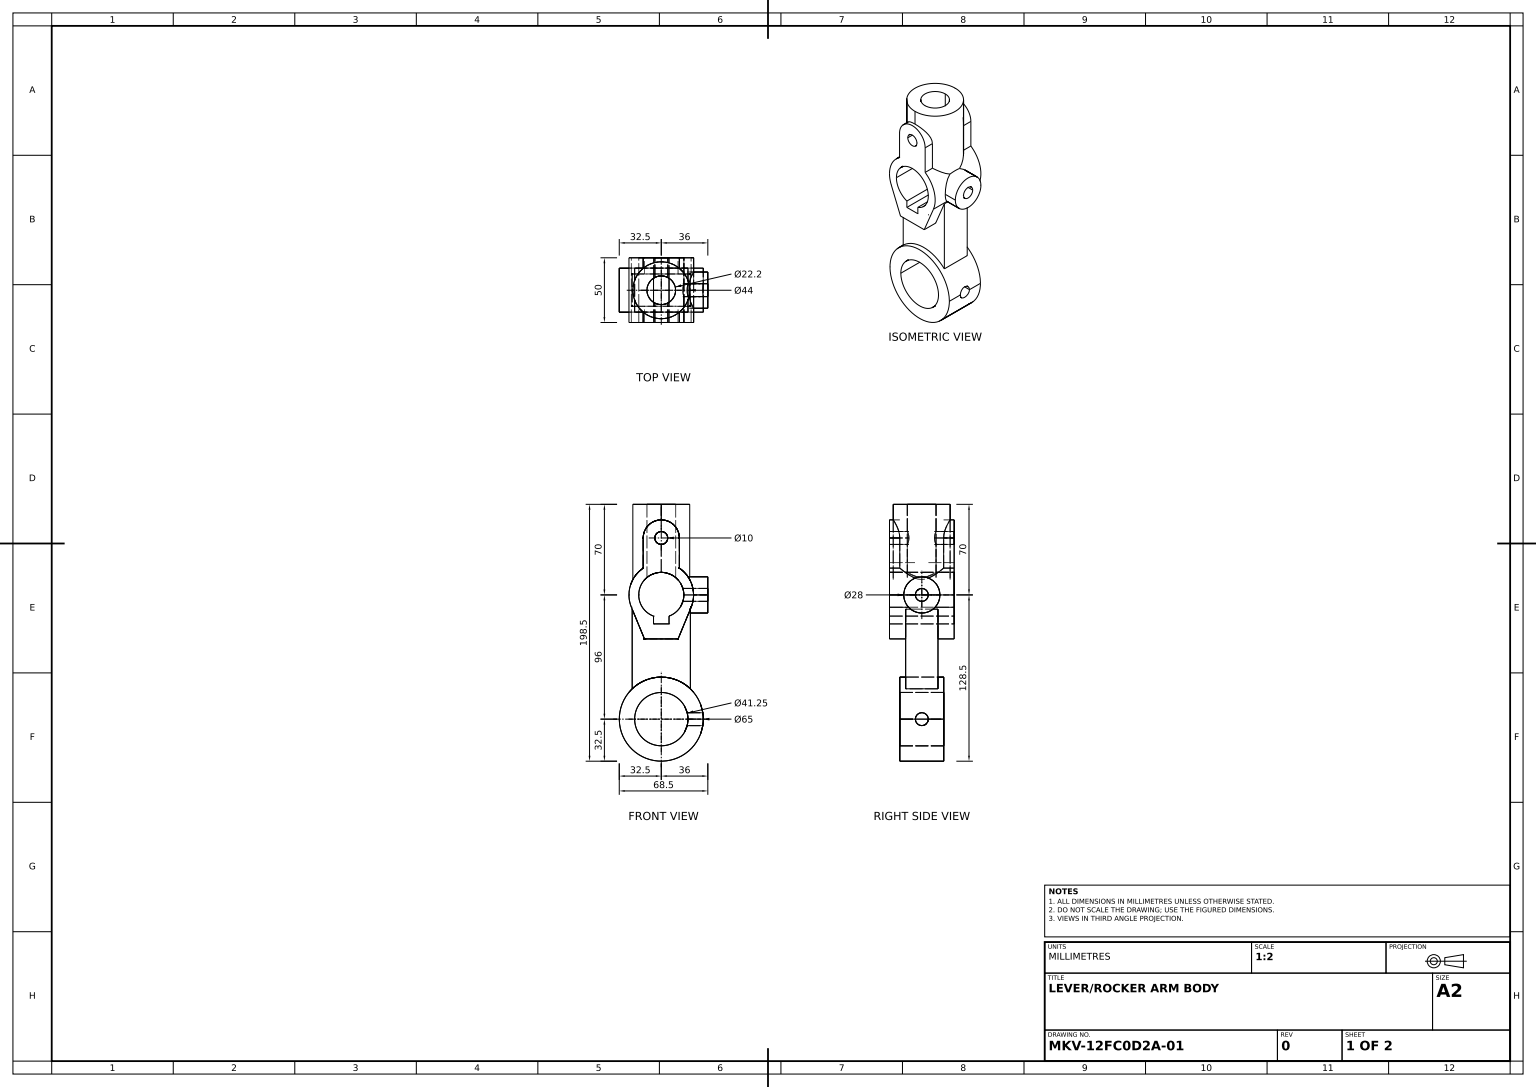
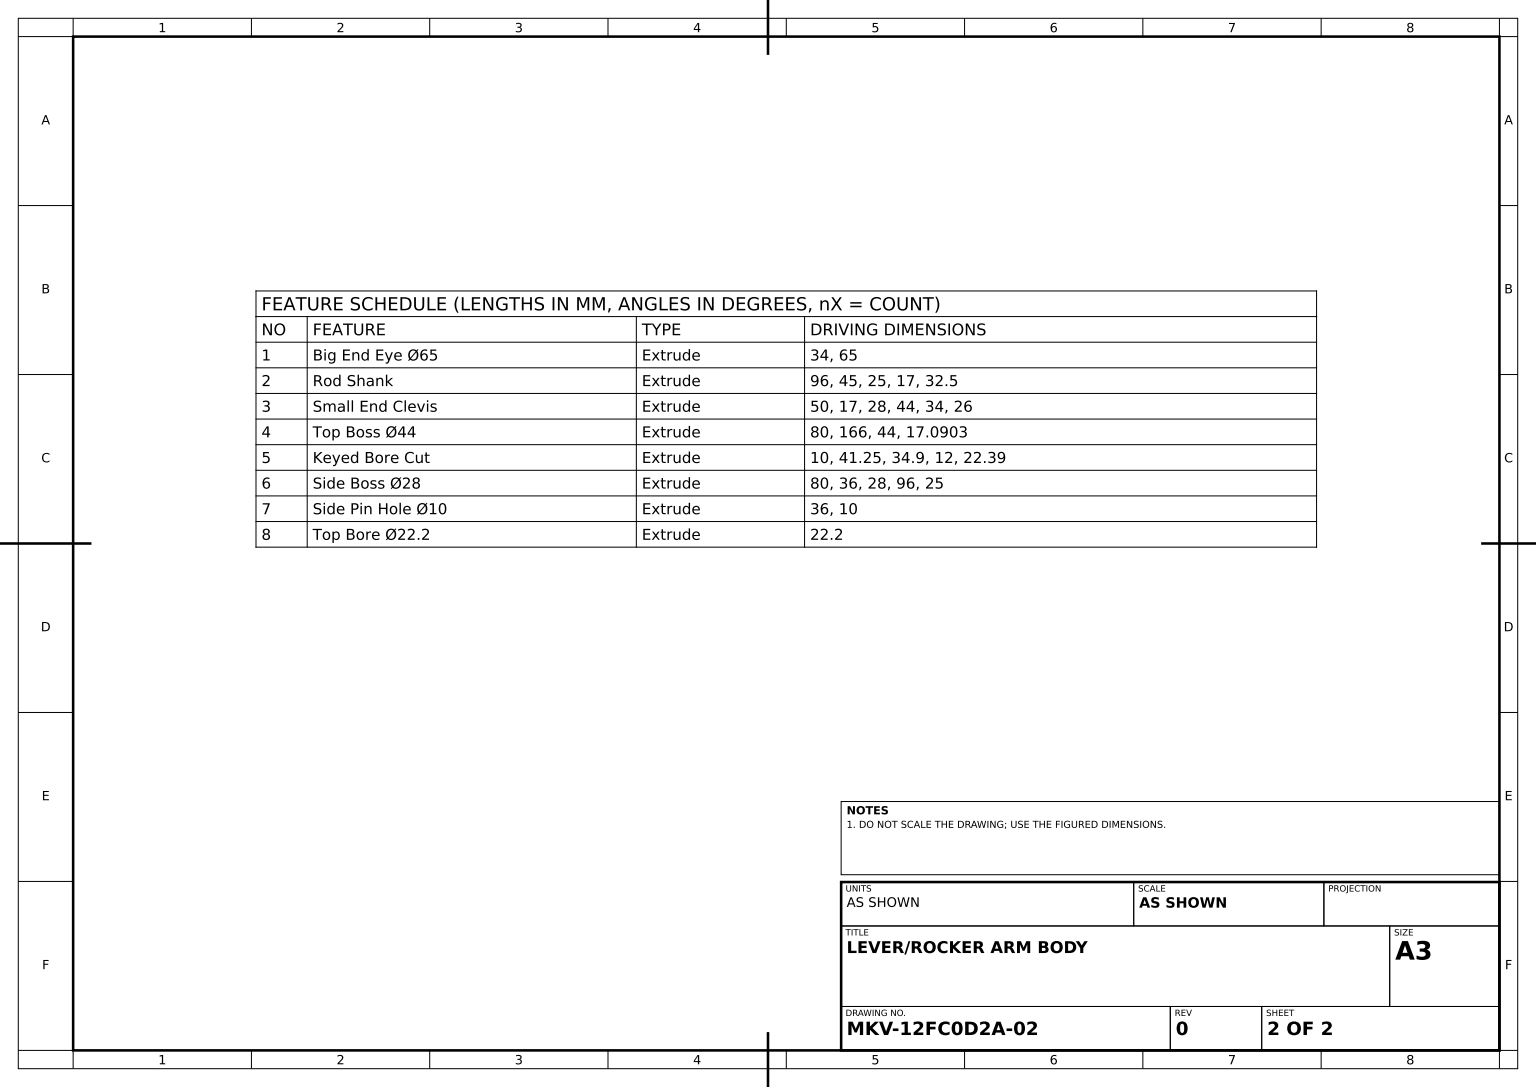
SolidWorks part; units mm, degrees
material "Plain Carbon Steel"
ref_plane "Front Plane" through (0, 0, 0) normal (0, 0, 1) x (1, 0, 0)
ref_plane "Top Plane" through (0, 0, 0) normal (0, 1, 0) x (1, 0, 0)
ref_plane "Right Plane" through (0, 0, 0) normal (1, 0, 0) x (0, 0, -1)
sketch "Big End Eye Sketch" plane through (0, 0, 0) normal (0, 0, 1) x (1, 0, 0)
  circle A0 centre (0, 0) radius 32.5
  dimension "D1" = 65
extrude "Big End Eye Ø65" add sketch "Big End Eye Sketch" along normal blind 34
sketch "Rod Shank Sketch" plane through (0, 0, 0) normal (0, 1, 0) x (1, 0, 0)
  line L1 (-22.5, -29.5) -> (22.5, -29.5)
  line L2 (-22.5, -29.5) -> (-22.5, -4.5)
  line L3 (-22.5, -4.5) -> (22.5, -4.5)
  line L4 (22.5, -29.5) -> (22.5, -4.5)
  line L5 (-22.5, -29.5) -> (22.5, -4.5) construction
  line L6 (-22.5, -4.5) -> (22.5, -29.5) construction
  line L8 (-32.5, 0) -> (-32.5, -34) construction
  point P0 (0, -17)
  dimension "D1" = 45
  dimension "D2" = 25
  dimension "D3" = 17
  dimension "D4" = 32.5
extrude "Rod Shank" add sketch "Rod Shank Sketch" along normal blind 96
sketch "Small End Clevis Sketch" plane through (0, 0, 0) normal (0, 0, 1) x (1, 0, 0)
  line L1 (-22.5, 96) -> (22.5, 96) construction
  line L2 (-14, 140) -> (-14, 116.7123)
  line L3 (14, 140) -> (14, 116.7123)
  line L4 (0, 0) -> (0, 62) construction
  line L5 (-13, 62) -> (13, 62)
  line L6 (13, 62) -> (23.1048, 86.4518)
  line L7 (-13, 62) -> (-23.1048, 86.4518)
  arc A2 (-14, 116.7123) -> (-23.1048, 86.4518) centre (0, 96) ccw
  arc A3 (14, 140) -> (-14, 140) centre (0, 140) ccw
  arc A4 (23.1048, 86.4518) -> (14, 116.7123) centre (0, 96) ccw
  point P18 (0, 62)
  dimension "D1" = 50
  dimension "D2" = 28
  dimension "D3" = 44
  dimension "D4" = 34
  dimension "D5" = 26
extrude "Small End Clevis" add sketch "Small End Clevis Sketch" along normal mid plane 50 from offset 17
sketch "Top Boss Sketch" plane through (0, 0, 0) normal (0, 1, 0) x (1, 0, 0)
  circle A0 centre (0, -17.0903) radius 22
  dimension "D1" = 44
  dimension "D2" = 17.0903
extrude "Top Boss Ø44" add sketch "Top Boss Sketch" against normal blind 80 from offset 166
sketch "Keyed Bore Sketch" plane through (0, 0, -8) normal (0, 0, -1) x (-1, 0, 0)
  line L2 (-6, 79.614) -> (-6, 73.61)
  line L3 (-6, 73.61) -> (6, 73.61)
  line L4 (6, 79.614) -> (6, 73.61)
  line L5 (0, 78.55) -> (6, 73.61) construction
  line L6 (-6, 73.61) -> (0, 78.55) construction
  circle A0 centre (0, 0) radius 20.625
  arc A1 (6, 79.614) -> (-6, 79.614) centre (0, 96) ccw
  circle A2 centre (0, 140) radius 5
  point P9 (0, 78.55)
  dimension "D1" = 10
  dimension "D2" = 41.25
  dimension "D3" = 34.9
  dimension "D4" = 12
  dimension "D5" = 22.39
extrude "Keyed Bore Cut" cut sketch "Keyed Bore Sketch" against normal through all
sketch "Side Boss Sketch" plane through (0, 0, 0) normal (1, 0, 0) x (0, 0, -1)
  line L0 (-42, 116.7123) -> (-42, 86.4518) construction
  circle A0 centre (-17, 96) radius 14
  dimension "D1" = 28
  dimension "D2" = 96
  dimension "D3" = 25
extrude "Side Boss Ø28" add sketch "Side Boss Sketch" against normal up to body from offset 36
sketch "Side Pin Hole Sketch" plane through (36, 0, 0) normal (1, 0, 0) x (0, 0, -1)
  circle A0 centre (-17, 96) radius 5
  circle A1 centre (-17, 0) radius 5
  dimension "D1" = 10
extrude "Side Pin Hole Ø10" cut sketch "Side Pin Hole Sketch" against normal blind 36
sketch "Top Bore Sketch" plane through (0, 166, 0) normal (0, 1, 0) x (1, 0, 0)
  circle A0 centre (0, -17.0903) radius 11.1
  dimension "D1" = 22.2
extrude "Top Bore Ø22.2" cut sketch "Top Bore Sketch" against normal up to surface (52.55 mm away)
